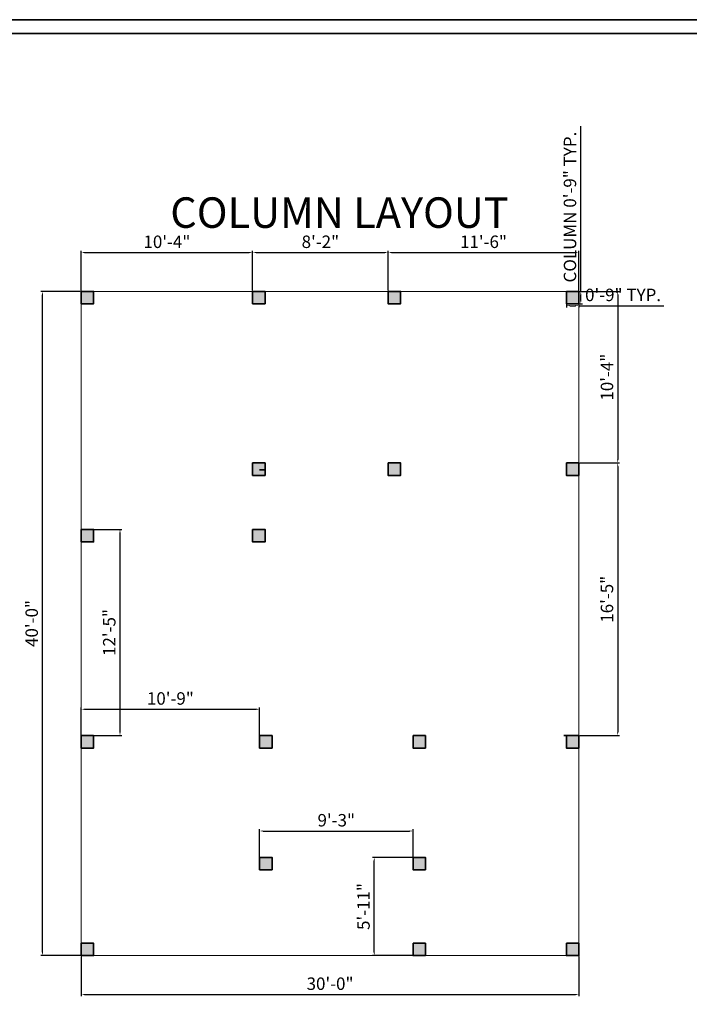
# Model space of a CAD drawing. Units: inches. Extents: x 2413 to 4117, y 1127 to 2321.
# Tile 4 of 5: x 3039 to 3524, y 1610 to 2321. Entities that reach past the tile are written whole.
import ezdxf

# ---------------------------------------------------------------- set-up
doc = ezdxf.new("R2010")
doc.units = ezdxf.units.IN
doc.linetypes.add('ACAD_ISO03W100', pattern=[30, 12, -18])
doc.layers.get('Defpoints').update_dxf_attribs({"linetype": 'ACAD_ISO03W100'})
for name, color, linetype, lineweight in [('A-ANNO-DIMS', 2, 'Continuous', 18), ('A-ANNO-TITL', 7, 'Continuous', 30), ('A-ANNO-TTLB', 7, 'Continuous', 35), ('S-COLS', 1, 'Continuous', 35), ('S-PLAN-REF', 8, 'Continuous', 18)]:
    doc.layers.add(name, color=color, linetype=linetype, lineweight=lineweight)
doc.styles.get("Standard").update_dxf_attribs({"font": 'arial.ttf'})
doc.dimstyles.new('ISO-25', dxfattribs={"dimtxt": 9, "dimasz": 2.5, "dimexe": 1.25, "dimexo": 0.625, "dimgap": 2, "dimtad": 1, "dimdec": 1, "dimlunit": 4, "dimtxsty": 'Standard', "dimcen": 2.5, "dimazin": 0, "dimtfac": 1, "dimtdec": 1, "dimtmove": 0, "dimatfit": 3, "dimfxl": 1, "dimarcsym": 0})

# ---------------------------------------------------------------- blocks, each defined once
blk = doc.blocks.new('COLUMN')
h = blk.add_hatch(color=256)
h.dxf.hatch_style = 1
h.paths.add_polyline_path([(3657.02, 1935.41), (3666.02, 1935.41), (3666.02, 1944.41), (3657.02, 1944.41)])
blk.add_lwpolyline([(3657.02, 1944.41), (3666.02, 1944.41), (3666.02, 1935.41), (3657.02, 1935.41)], close=True)
blk = doc.blocks.new('*D14')
at = {"layer": 'A-ANNO-DIMS', "color": 0, "lineweight": -2, "transparency": 16777216}
for p, q in [((3445.09, 2125.03), (3445.09, 2244.27)), ((3444.37, 2125.03), (3446.34, 2125.03)), ((3445.09, 2118.53), (3445.09, 2122.53)), ((3444.37, 2116.03), (3446.34, 2116.03))]:
    blk.add_line(p, q, dxfattribs=at)
at = {"layer": 'A-ANNO-DIMS', "color": 0, "transparency": 16777216}
for points in [[(3444.68, 2122.53), (3445.51, 2122.53), (3445.09, 2125.03)], [(3444.68, 2118.53), (3445.51, 2118.53), (3445.09, 2116.03)]]:
    blk.add_solid(points, dxfattribs=at)
at = {"layer": 'Defpoints', "color": 0, "transparency": 16777216}
for p in [(3443.74, 2125.03), (3445.09, 2125.03), (3443.74, 2116.03)]:
    blk.add_point(p, dxfattribs=at)
at = {"layer": 'A-ANNO-DIMS', "color": 0, "transparency": 16777216, "insert": (3438.44, 2185.9), "char_height": 9, "attachment_point": 5, "rotation": 90}
blk.add_mtext('COLUMN 0\'-9" TYP.', dxfattribs=at)
blk = doc.blocks.new('*D15')
at = {"layer": 'A-ANNO-DIMS', "color": 0, "lineweight": -2, "transparency": 16777216}
for p, q in [((3434.74, 2115.41), (3434.74, 2113.43)), ((3437.24, 2114.68), (3441.24, 2114.68)), ((3443.74, 2115.41), (3443.74, 2113.43)), ((3443.74, 2114.68), (3505.1, 2114.68))]:
    blk.add_line(p, q, dxfattribs=at)
at = {"layer": 'A-ANNO-DIMS', "color": 0, "transparency": 16777216}
for points in [[(3437.24, 2115.1), (3437.24, 2114.27), (3434.74, 2114.68)], [(3441.24, 2115.1), (3441.24, 2114.27), (3443.74, 2114.68)]]:
    blk.add_solid(points, dxfattribs=at)
at = {"layer": 'Defpoints', "color": 0, "transparency": 16777216}
for p in [(3434.74, 2116.03), (3443.74, 2116.03), (3443.74, 2114.68)]:
    blk.add_point(p, dxfattribs=at)
at = {"layer": 'A-ANNO-DIMS', "color": 0, "transparency": 16777216, "insert": (3475.67, 2121.28), "char_height": 9, "attachment_point": 5}
blk.add_mtext('0\'-9" TYP.', dxfattribs=at)
blk = doc.blocks.new('*D43')
at = {"layer": 'A-ANNO-DIMS', "color": 0, "lineweight": -2, "transparency": 16777216}
for p, q in [((3083.74, 2125.66), (3083.74, 2154.33)), ((3086.24, 2153.08), (3205.24, 2153.08)), ((3207.74, 2125.66), (3207.74, 2154.33))]:
    blk.add_line(p, q, dxfattribs=at)
at = {"layer": 'A-ANNO-DIMS', "color": 0, "transparency": 16777216}
for points in [[(3086.24, 2153.5), (3086.24, 2152.67), (3083.74, 2153.08)], [(3205.24, 2153.5), (3205.24, 2152.67), (3207.74, 2153.08)]]:
    blk.add_solid(points, dxfattribs=at)
at = {"layer": 'Defpoints', "color": 0, "transparency": 16777216}
for p in [(3207.74, 2153.08), (3083.74, 2125.03), (3207.74, 2125.03)]:
    blk.add_point(p, dxfattribs=at)
at = {"layer": 'A-ANNO-DIMS', "color": 0, "transparency": 16777216, "insert": (3145.74, 2159.68), "char_height": 9, "attachment_point": 5}
blk.add_mtext('10\'-4"', dxfattribs=at)
blk = doc.blocks.new('*D44')
at = {"layer": 'A-ANNO-DIMS', "color": 0, "lineweight": -2, "transparency": 16777216}
for p, q in [((3207.74, 2125.66), (3207.74, 2154.33)), ((3210.24, 2153.08), (3303.24, 2153.08)), ((3305.74, 2125.66), (3305.74, 2154.33))]:
    blk.add_line(p, q, dxfattribs=at)
at = {"layer": 'A-ANNO-DIMS', "color": 0, "transparency": 16777216}
for points in [[(3210.24, 2153.5), (3210.24, 2152.67), (3207.74, 2153.08)], [(3303.24, 2153.5), (3303.24, 2152.67), (3305.74, 2153.08)]]:
    blk.add_solid(points, dxfattribs=at)
at = {"layer": 'Defpoints', "color": 0, "transparency": 16777216}
for p in [(3305.74, 2153.08), (3207.74, 2125.03), (3305.74, 2125.03)]:
    blk.add_point(p, dxfattribs=at)
at = {"layer": 'A-ANNO-DIMS', "color": 0, "transparency": 16777216, "insert": (3256.74, 2159.68), "char_height": 9, "attachment_point": 5}
blk.add_mtext('8\'-2"', dxfattribs=at)
blk = doc.blocks.new('*D45')
at = {"layer": 'A-ANNO-DIMS', "color": 0, "lineweight": -2, "transparency": 16777216}
for p, q in [((3305.74, 2125.66), (3305.74, 2154.33)), ((3308.24, 2153.08), (3441.24, 2153.08)), ((3443.74, 2125.66), (3443.74, 2154.33))]:
    blk.add_line(p, q, dxfattribs=at)
at = {"layer": 'A-ANNO-DIMS', "color": 0, "transparency": 16777216}
for points in [[(3308.24, 2153.5), (3308.24, 2152.67), (3305.74, 2153.08)], [(3441.24, 2153.5), (3441.24, 2152.67), (3443.74, 2153.08)]]:
    blk.add_solid(points, dxfattribs=at)
at = {"layer": 'Defpoints', "color": 0, "transparency": 16777216}
for p in [(3443.74, 2153.08), (3305.74, 2125.03), (3443.74, 2125.03)]:
    blk.add_point(p, dxfattribs=at)
at = {"layer": 'A-ANNO-DIMS', "color": 0, "transparency": 16777216, "insert": (3374.74, 2159.68), "char_height": 9, "attachment_point": 5}
blk.add_mtext('11\'-6"', dxfattribs=at)
blk = doc.blocks.new('*D46')
at = {"layer": 'A-ANNO-DIMS', "color": 0, "lineweight": -2, "transparency": 16777216}
for p, q in [((3083.74, 1795.66), (3083.74, 1824.33)), ((3086.24, 1823.08), (3210.24, 1823.08)), ((3212.74, 1795.66), (3212.74, 1824.33))]:
    blk.add_line(p, q, dxfattribs=at)
at = {"layer": 'A-ANNO-DIMS', "color": 0, "transparency": 16777216}
for points in [[(3086.24, 1823.5), (3086.24, 1822.67), (3083.74, 1823.08)], [(3210.24, 1823.5), (3210.24, 1822.67), (3212.74, 1823.08)]]:
    blk.add_solid(points, dxfattribs=at)
at = {"layer": 'Defpoints', "color": 0, "transparency": 16777216}
for p in [(3212.74, 1823.08), (3083.74, 1795.03), (3212.74, 1795.03)]:
    blk.add_point(p, dxfattribs=at)
at = {"layer": 'A-ANNO-DIMS', "color": 0, "transparency": 16777216, "insert": (3148.24, 1829.68), "char_height": 9, "attachment_point": 5}
blk.add_mtext('10\'-9"', dxfattribs=at)
blk = doc.blocks.new('*D47')
at = {"layer": 'A-ANNO-DIMS', "color": 0, "lineweight": -2, "transparency": 16777216}
for p, q in [((3212.74, 1707.66), (3212.74, 1736.33)), ((3323.74, 1707.66), (3323.74, 1736.33)), ((3215.24, 1735.08), (3321.24, 1735.08))]:
    blk.add_line(p, q, dxfattribs=at)
at = {"layer": 'A-ANNO-DIMS', "color": 0, "transparency": 16777216}
for points in [[(3215.24, 1735.5), (3215.24, 1734.67), (3212.74, 1735.08)], [(3321.24, 1735.5), (3321.24, 1734.67), (3323.74, 1735.08)]]:
    blk.add_solid(points, dxfattribs=at)
at = {"layer": 'Defpoints', "color": 0, "transparency": 16777216}
for p in [(3323.74, 1735.08), (3212.74, 1707.03), (3323.74, 1707.03)]:
    blk.add_point(p, dxfattribs=at)
at = {"layer": 'A-ANNO-DIMS', "color": 0, "transparency": 16777216, "insert": (3268.24, 1741.68), "char_height": 9, "attachment_point": 5}
blk.add_mtext('9\'-3"', dxfattribs=at)
blk = doc.blocks.new('*D48')
at = {"layer": 'A-ANNO-DIMS', "color": 0, "lineweight": -2, "transparency": 16777216}
for p, q in [((3444.37, 2125.03), (3473.04, 2125.03)), ((3471.79, 2122.53), (3471.79, 2003.53)), ((3444.37, 2001.03), (3473.04, 2001.03))]:
    blk.add_line(p, q, dxfattribs=at)
at = {"layer": 'A-ANNO-DIMS', "color": 0, "transparency": 16777216}
for points in [[(3471.38, 2122.53), (3472.21, 2122.53), (3471.79, 2125.03)], [(3471.38, 2003.53), (3472.21, 2003.53), (3471.79, 2001.03)]]:
    blk.add_solid(points, dxfattribs=at)
at = {"layer": 'Defpoints', "color": 0, "transparency": 16777216}
for p in [(3443.74, 2125.03), (3443.74, 2001.03), (3471.79, 2001.03)]:
    blk.add_point(p, dxfattribs=at)
at = {"layer": 'A-ANNO-DIMS', "color": 0, "transparency": 16777216, "insert": (3465.2, 2063.03), "char_height": 9, "attachment_point": 5, "rotation": 90}
blk.add_mtext('10\'-4"', dxfattribs=at)
blk = doc.blocks.new('*D49')
at = {"layer": 'A-ANNO-DIMS', "color": 0, "lineweight": -2, "transparency": 16777216}
for p, q in [((3444.37, 2001.03), (3473.04, 2001.03)), ((3471.79, 1998.53), (3471.79, 1806.53)), ((3444.37, 1804.03), (3473.04, 1804.03))]:
    blk.add_line(p, q, dxfattribs=at)
at = {"layer": 'A-ANNO-DIMS', "color": 0, "transparency": 16777216}
for points in [[(3471.38, 1998.53), (3472.21, 1998.53), (3471.79, 2001.03)], [(3471.38, 1806.53), (3472.21, 1806.53), (3471.79, 1804.03)]]:
    blk.add_solid(points, dxfattribs=at)
at = {"layer": 'Defpoints', "color": 0, "transparency": 16777216}
for p in [(3443.74, 2001.03), (3443.74, 1804.03), (3471.79, 1804.03)]:
    blk.add_point(p, dxfattribs=at)
at = {"layer": 'A-ANNO-DIMS', "color": 0, "transparency": 16777216, "insert": (3465.2, 1902.53), "char_height": 9, "attachment_point": 5, "rotation": 90}
blk.add_mtext('16\'-5"', dxfattribs=at)
blk = doc.blocks.new('*D50')
at = {"layer": 'A-ANNO-DIMS', "color": 0, "lineweight": -2, "transparency": 16777216}
for p, q in [((3084.37, 1953.03), (3113.04, 1953.03)), ((3111.79, 1950.53), (3111.79, 1806.53)), ((3084.37, 1804.03), (3113.04, 1804.03))]:
    blk.add_line(p, q, dxfattribs=at)
at = {"layer": 'A-ANNO-DIMS', "color": 0, "transparency": 16777216}
for points in [[(3111.38, 1950.53), (3112.21, 1950.53), (3111.79, 1953.03)], [(3111.38, 1806.53), (3112.21, 1806.53), (3111.79, 1804.03)]]:
    blk.add_solid(points, dxfattribs=at)
at = {"layer": 'Defpoints', "color": 0, "transparency": 16777216}
for p in [(3083.74, 1953.03), (3083.74, 1804.03), (3111.79, 1804.03)]:
    blk.add_point(p, dxfattribs=at)
at = {"layer": 'A-ANNO-DIMS', "color": 0, "transparency": 16777216, "insert": (3105.2, 1878.53), "char_height": 9, "attachment_point": 5, "rotation": 90}
blk.add_mtext('12\'-5"', dxfattribs=at)
blk = doc.blocks.new('*D51')
at = {"layer": 'A-ANNO-DIMS', "color": 0, "lineweight": -2, "transparency": 16777216}
for p, q in [((3323.12, 1716.03), (3294.44, 1716.03)), ((3295.69, 1647.53), (3295.69, 1713.53)), ((3323.12, 1645.03), (3294.44, 1645.03))]:
    blk.add_line(p, q, dxfattribs=at)
at = {"layer": 'A-ANNO-DIMS', "color": 0, "transparency": 16777216}
for points in [[(3295.28, 1713.53), (3296.11, 1713.53), (3295.69, 1716.03)], [(3295.28, 1647.53), (3296.11, 1647.53), (3295.69, 1645.03)]]:
    blk.add_solid(points, dxfattribs=at)
at = {"layer": 'Defpoints', "color": 0, "transparency": 16777216}
for p in [(3295.69, 1716.03), (3323.74, 1716.03), (3323.74, 1645.03)]:
    blk.add_point(p, dxfattribs=at)
at = {"layer": 'A-ANNO-DIMS', "color": 0, "transparency": 16777216, "insert": (3289.1, 1680.53), "char_height": 9, "attachment_point": 5, "rotation": 90}
blk.add_mtext('5\'-11"', dxfattribs=at)
blk = doc.blocks.new('*D52')
at = {"layer": 'A-ANNO-DIMS', "color": 0, "lineweight": -2, "transparency": 16777216}
for p, q in [((3083.74, 1644.41), (3083.74, 1615.73)), ((3443.74, 1644.41), (3443.74, 1615.73)), ((3086.24, 1616.98), (3441.24, 1616.98))]:
    blk.add_line(p, q, dxfattribs=at)
at = {"layer": 'A-ANNO-DIMS', "color": 0, "transparency": 16777216}
for points in [[(3086.24, 1617.4), (3086.24, 1616.57), (3083.74, 1616.98)], [(3441.24, 1617.4), (3441.24, 1616.57), (3443.74, 1616.98)]]:
    blk.add_solid(points, dxfattribs=at)
at = {"layer": 'Defpoints', "color": 0, "transparency": 16777216}
for p in [(3083.74, 1645.03), (3443.74, 1645.03), (3443.74, 1616.98)]:
    blk.add_point(p, dxfattribs=at)
at = {"layer": 'A-ANNO-DIMS', "color": 0, "transparency": 16777216, "insert": (3263.74, 1623.58), "char_height": 9, "attachment_point": 5}
blk.add_mtext('30\'-0"', dxfattribs=at)
blk = doc.blocks.new('*D53')
at = {"layer": 'A-ANNO-DIMS', "color": 0, "lineweight": -2, "transparency": 16777216}
for p, q in [((3083.12, 2125.03), (3054.44, 2125.03)), ((3055.69, 1647.53), (3055.69, 2122.53)), ((3083.12, 1645.03), (3054.44, 1645.03))]:
    blk.add_line(p, q, dxfattribs=at)
at = {"layer": 'A-ANNO-DIMS', "color": 0, "transparency": 16777216}
for points in [[(3055.28, 2122.53), (3056.11, 2122.53), (3055.69, 2125.03)], [(3055.28, 1647.53), (3056.11, 1647.53), (3055.69, 1645.03)]]:
    blk.add_solid(points, dxfattribs=at)
at = {"layer": 'Defpoints', "color": 0, "transparency": 16777216}
for p in [(3055.69, 2125.03), (3083.74, 2125.03), (3083.74, 1645.03)]:
    blk.add_point(p, dxfattribs=at)
at = {"layer": 'A-ANNO-DIMS', "color": 0, "transparency": 16777216, "insert": (3049.1, 1885.03), "char_height": 9, "attachment_point": 5, "rotation": 90}
blk.add_mtext('40\'-0"', dxfattribs=at)

msp = doc.modelspace()

# ---------------------------------------------------------------- linework, layer by layer
at = {"layer": 'A-ANNO-TTLB'}
for points in [[(2412.62, 2321.32), (4117.04, 2321.32), (4117.04, 1126.9), (2412.62, 1126.9)], [(2422.62, 2311.32), (4107.04, 2311.32), (4107.04, 1136.9), (2422.62, 1136.9)]]:
    msp.add_lwpolyline(points, close=True, dxfattribs=at)
at = {"layer": 'S-COLS'}
for p, q in [((3212.74, 1996.03), (3216.74, 1996.03)), ((3216.74, 1992.03), (3216.74, 1996.03)), ((3216.74, 1950.03), (3216.74, 1944.03)), ((3216.74, 1944.03), (3216.74, 1950.03)), ((3323.74, 1804.03), (3323.74, 1800.03)), ((3432.74, 1804.03), (3434.74, 1804.03)), ((3323.74, 1645.03), (3323.74, 1654.03)), ((3332.74, 1645.03), (3332.74, 1654.03))]:
    msp.add_line(p, q, dxfattribs=at)
at = {"layer": 'S-PLAN-REF'}
for p, q in [((3083.74, 2125.03), (3083.74, 1645.03)), ((3443.74, 2125.03), (3083.74, 2125.03)), ((3443.74, 1645.03), (3443.74, 2125.03)), ((3083.74, 1645.03), (3443.74, 1645.03))]:
    msp.add_line(p, q, dxfattribs=at)

# ---------------------------------------------------------------- block references
at = {"layer": 'S-COLS'}
for p in [(-573.27, 180.62), (-449.27, 180.62), (-351.27, 180.62), (-222.27, 180.62), (-449.27, 56.62), (-351.27, 56.62), (-222.27, 56.62), (-573.27, 8.62), (-449.27, 8.62), (-573.27, -140.38), (-444.27, -140.38), (-333.27, -140.38), (-222.27, -140.38), (-444.27, -228.38), (-333.27, -228.38), (-573.27, -290.38), (-333.27, -290.38), (-222.27, -290.38)]:
    msp.add_blockref('COLUMN', p, dxfattribs=at)

# ---------------------------------------------------------------- texts
at = {"layer": 'A-ANNO-TITL'}
msp.add_text('COLUMN LAYOUT', height=22.0248, dxfattribs=at).set_placement((3148.16, 2170.92))

# ---------------------------------------------------------------- dimensions: what is measured, and where the dimension line sits
at = {"layer": 'A-ANNO-DIMS'}
dim = msp.add_linear_dim(base=(3445.09, 2125.03), p1=(3443.74, 2116.03), p2=(3443.74, 2125.03), angle=90, text='COLUMN <> TYP.', dimstyle='ISO-25', override={"dimdec": 1, "dimlfac": 1, "dimrnd": 0, "dimzin": 1, "dimdsep": 46, "dimlunit": 4, "dimfrac": 2}, dxfattribs=at)
dim.commit()
dim.dimension.update_dxf_attribs({"geometry": '*D14', "text_midpoint": (3438.44, 2185.9)})
for base, p1, p2, picture, middle in [((3207.74, 2153.08), (3083.74, 2125.03), (3207.74, 2125.03), '*D43', (3145.74, 2159.68)), ((3305.74, 2153.08), (3207.74, 2125.03), (3305.74, 2125.03), '*D44', (3256.74, 2159.68)), ((3443.74, 2153.08), (3305.74, 2125.03), (3443.74, 2125.03), '*D45', (3374.74, 2159.68)), ((3212.74, 1823.08), (3083.74, 1795.03), (3212.74, 1795.03), '*D46', (3148.24, 1829.68)), ((3323.74, 1735.08), (3212.74, 1707.03), (3323.74, 1707.03), '*D47', (3268.24, 1741.68)), ((3443.74, 1616.98), (3083.74, 1645.03), (3443.74, 1645.03), '*D52', (3263.74, 1623.58))]:
    dim = msp.add_linear_dim(base=base, p1=p1, p2=p2, dimstyle='ISO-25', override={"dimdec": 1, "dimlfac": 1, "dimrnd": 0, "dimzin": 1, "dimdsep": 46, "dimlunit": 4, "dimfrac": 2}, dxfattribs=at)
    dim.commit()
    dim.dimension.update_dxf_attribs({"geometry": picture, "text_midpoint": middle})
dim = msp.add_linear_dim(base=(3443.74, 2114.68), p1=(3434.74, 2116.03), p2=(3443.74, 2116.03), text='<> TYP.', dimstyle='ISO-25', override={"dimdec": 1, "dimlfac": 1, "dimrnd": 0, "dimzin": 1, "dimdsep": 46, "dimlunit": 4, "dimfrac": 2}, dxfattribs=at)
dim.commit()
dim.dimension.update_dxf_attribs({"geometry": '*D15', "text_midpoint": (3475.67, 2121.28)})
for base, p1, p2, angle, picture, middle in [((3055.69, 2125.03), (3083.74, 1645.03), (3083.74, 2125.03), 90, '*D53', (3049.1, 1885.03)), ((3471.79, 2001.03), (3443.74, 2125.03), (3443.74, 2001.03), 90, '*D48', (3465.2, 2063.03)), ((3471.79, 1804.03), (3443.74, 2001.03), (3443.74, 1804.03), 90, '*D49', (3465.2, 1902.53)), ((3111.79, 1804.03), (3083.74, 1953.03), (3083.74, 1804.03), 270, '*D50', (3105.2, 1878.53)), ((3295.69, 1716.03), (3323.74, 1645.03), (3323.74, 1716.03), 90, '*D51', (3289.1, 1680.53))]:
    dim = msp.add_linear_dim(base=base, p1=p1, p2=p2, angle=angle, dimstyle='ISO-25', override={"dimdec": 1, "dimlfac": 1, "dimrnd": 0, "dimzin": 1, "dimdsep": 46, "dimlunit": 4, "dimfrac": 2}, dxfattribs=at)
    dim.commit()
    dim.dimension.update_dxf_attribs({"geometry": picture, "text_midpoint": middle})

doc.saveas('drawing.dxf')
